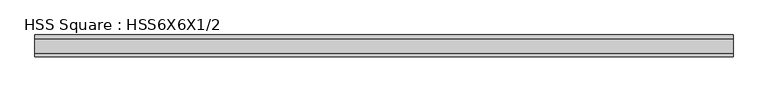
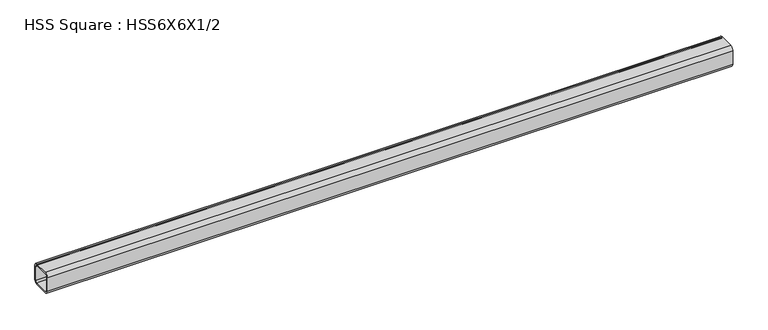
"""IFC4 building model written with IfcOpenShell, lengths in millimetres: member geometry, HSS Square : HSS6X6X1/2."""

from ifc_helpers import new_model, si_unit, point, frame, frame_2d, origin, place, context, project, spatial, polyline, circle_curve, trimmed, segment, composite_curve, outline, extrude, source, transform, mapped, element, save


def hss_square_hss6x6x1_2_7c43692b(model_context):
    return source(origin(), model_context, "Body", "SweptSolid", [
        extrude(outline(composite_curve([segment(polyline([(76.2, 50.8), (76.2, -50.8)]), True, "CONTINUOUS"), segment(trimmed(circle_curve(frame_2d((50.8, -50.8)), 25.4), [point((76.2, -50.8))], [point((50.8, -76.2))], False, "CARTESIAN"), True, "CONTINUOUS"), segment(polyline([(50.8, -76.2), (-50.8, -76.2)]), True, "CONTINUOUS"), segment(trimmed(circle_curve(frame_2d((-50.8, -50.8)), 25.4), [point((-50.8, -76.2))], [point((-76.2, -50.8))], False, "CARTESIAN"), True, "CONTINUOUS"), segment(polyline([(-76.2, -50.8), (-76.2, 50.8)]), True, "CONTINUOUS"), segment(trimmed(circle_curve(frame_2d((-50.8, 50.8)), 25.4), [point((-76.2, 50.8))], [point((-50.8, 76.2))], False, "CARTESIAN"), True, "CONTINUOUS"), segment(polyline([(-50.8, 76.2), (50.8, 76.2)]), True, "CONTINUOUS"), segment(trimmed(circle_curve(frame_2d((50.8, 50.8)), 25.4), [point((50.8, 76.2))], [point((76.2, 50.8))], False, "CARTESIAN"), True, "CONTINUOUS")], self_intersect=False), holes=[composite_curve([segment(trimmed(circle_curve(frame_2d((-50.8, 50.8)), 12.7), [point((-50.8, 63.5))], [point((-63.5, 50.8))], True, "CARTESIAN"), True, "CONTINUOUS"), segment(polyline([(-63.5, 50.8), (-63.5, -50.8)]), True, "CONTINUOUS"), segment(trimmed(circle_curve(frame_2d((-50.8, -50.8)), 12.7), [point((-63.5, -50.8))], [point((-50.8, -63.5))], True, "CARTESIAN"), True, "CONTINUOUS"), segment(polyline([(-50.8, -63.5), (50.8, -63.5)]), True, "CONTINUOUS"), segment(trimmed(circle_curve(frame_2d((50.8, -50.8)), 12.7), [point((50.8, -63.5))], [point((63.5, -50.8))], True, "CARTESIAN"), True, "CONTINUOUS"), segment(polyline([(63.5, -50.8), (63.5, 50.8)]), True, "CONTINUOUS"), segment(trimmed(circle_curve(frame_2d((50.8, 50.8)), 12.7), [point((63.5, 50.8))], [point((50.8, 63.5))], True, "CARTESIAN"), True, "CONTINUOUS"), segment(polyline([(50.8, 63.5), (-50.8, 63.5)]), True, "CONTINUOUS")], self_intersect=False)]), frame((-2376.9834929, 0.0, 0.0), z_axis=(1.0, 0.0, 0.0), x_axis=(0.0, 1.0, 0.0)), (0.0, 0.0, 1.0), 4840.8896454),
    ])


if __name__ == "__main__":
    model = new_model("IFC4")
    model_context = context("Model", 3, world=origin())
    ifc_project = project(units=[si_unit("LENGTHUNIT", "METRE", prefix="MILLI")], contexts=[model_context])
    site = spatial("IfcSite", under=ifc_project)
    building = spatial("IfcBuilding", under=site)
    placement = place(None, origin())
    hss_square_hss6x6x1_2_shape = hss_square_hss6x6x1_2_7c43692b(model_context)
    element("IfcMember", 1, ObjectType="HSS Square : HSS6X6X1/2", at=placement, inside=building, context=model_context, shape_type="MappedRepresentation", body=[
        mapped(hss_square_hss6x6x1_2_shape, transform((0.0, 0.0, 0.0), x_axis=(1.0, 0.0, 0.0), y_axis=(0.0, 1.0, 0.0), z_axis=(0.0, 0.0, 1.0))),
    ])
    save(model, "model.ifc")

# Revit data of these elements
# Type "HSS Square : HSS6X6X1/2"
#   Section Name Key = "HSS 6X6X1/2"
#   Assembly Code = "B10"
#   Width = 6.000"
#   Wall Nominal Thickness = 0.500"
#   Wall Design Thickness = 0.465"
#   Torsional Moment of Inertia = 81.10 in⁴
#   Torsional Modulus = 28.10 in³
#   Section Area = 9.74 in²
#   Plastic Modulus weak axis = 19.80 in³
#   Plastic Modulus strong axis = 19.80 in³
#   Outer Fillet = 1.000"
#   Nominal Weight = 35.24 lbf/ft
#   Moment of Inertia weak axis = 48.30 in⁴
#   Moment of Inertia strong axis = 48.30 in⁴
#   Inner Fillet = 0.500"
#   Height = 6.000"
#   Elastic Modulus weak axis = 16.10 in³
#   Elastic Modulus strong axis = 16.10 in³
#   Centroid Vertical = 3.000"
#   Centroid Horizontal = 3.000"
#   Length [instance default] = 5' - 0"
#   Structural Material [instance default] = Steel ASTM A500, Grade B, Rectangular and Square
#   Principal Axes Angle = 0
# Element 1 (IfcMember, "HSS Square : HSS6X6X1/2")
#   Structural Material = Steel ASTM A992
#   Materials on its faces: "Steel ASTM A992"
# Materials
#   "Steel ASTM A500, Grade B, Rectangular and Square": class "Metal", colour RGB 199 199 199, transparency 0, Description = "Carbon steel", Cost = 0
#   "Steel ASTM A992": class "Metal", colour RGB 199 199 199, transparency 0, Description = "Structural steel 50ksi", Cost = 0
